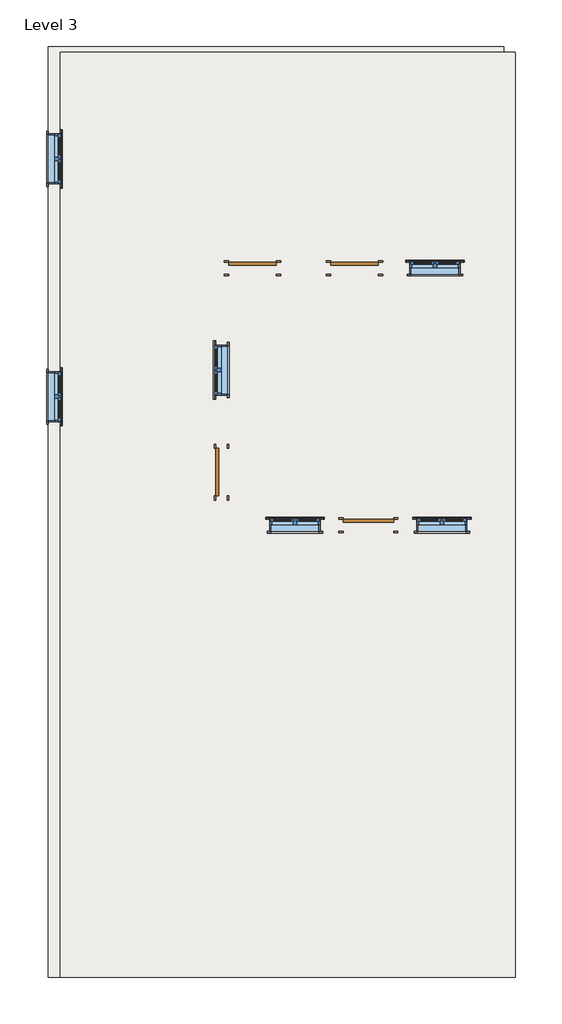
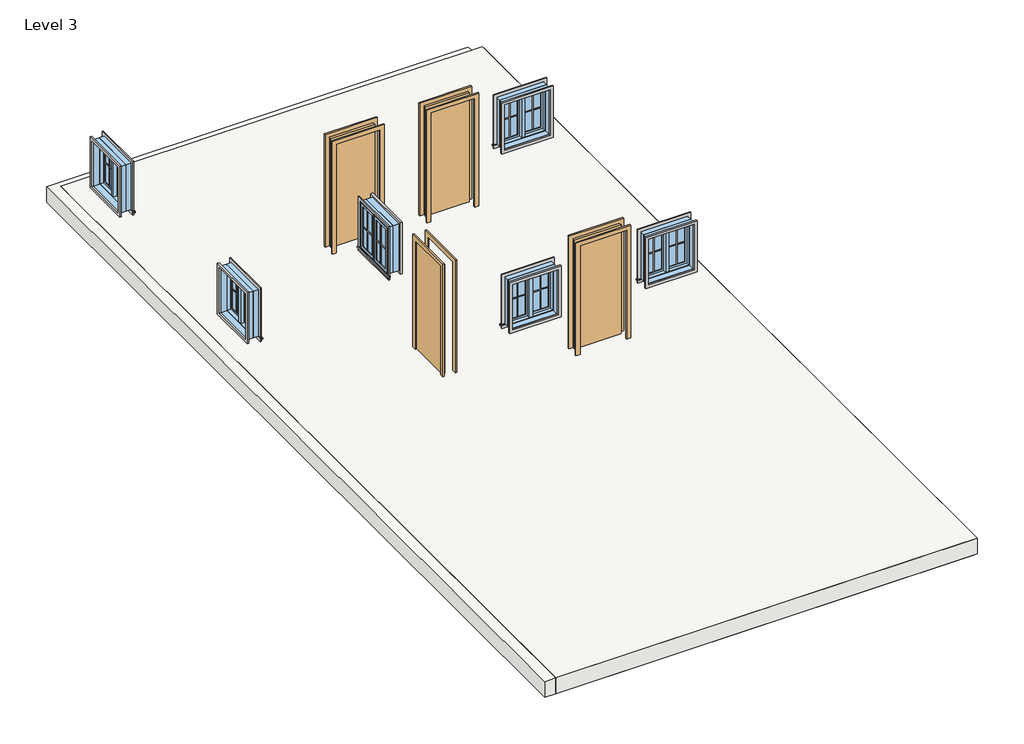
# One storey: 24 proxies, 6 windows, 4 doors, 4 slabs.
"""IFC4 building model written with IfcOpenShell, lengths in millimetres."""

from ifc_helpers import new_model, si_unit, frame, origin, place, context, project, spatial, polyline, outline, extrude, faceted_brep, transform, mapped, element, save
from components import muntin_pattern_2x2_muntin_pattern_2x2_b3fe6957, muntin_pattern_2x2_muntin_pattern_2x2_3e0ecaf2, trim_window_exterior_flat_with_sill_41619996, trim_window_interior_flat_picture_frame_51c85655, door_64d5ae29, door_f75d31f8, window_c29befe5

model = new_model("IFC4")

# Units and contexts
model_context = context("Model", 3, world=origin())
ifc_project = project(units=[si_unit("LENGTHUNIT", "METRE", prefix="MILLI")], contexts=[model_context])

# Site, building, storey
site = spatial("IfcSite", under=ifc_project)
building = spatial("IfcBuilding", under=site)
storey = spatial("IfcBuildingStorey", under=building, Name="Level 3", Elevation=12801.6)

# Proxies
placement = place(None, origin())
muntin_pattern_2x2_muntin_pattern_2x2_shape = muntin_pattern_2x2_muntin_pattern_2x2_b3fe6957(model_context)
element("IfcBuildingElementProxy", 1, Name="Muntin Pattern_2x2 : Muntin Pattern_2x2", ObjectType="Muntin Pattern_2x2 : Muntin Pattern_2x2", at=placement, inside=storey, context=model_context, shape_type="MappedRepresentation", body=[
    mapped(muntin_pattern_2x2_muntin_pattern_2x2_shape, transform((-15829.9638186, 14328.8576951, 13785.85), x_axis=(0.0, -1.0, 0.0), y_axis=(1.0, 0.0, 0.0), z_axis=(0.0, 0.0, 1.0))),
])
element("IfcBuildingElementProxy", 2, Name="Muntin Pattern_2x2 : Muntin Pattern_2x2", ObjectType="Muntin Pattern_2x2 : Muntin Pattern_2x2", at=placement, inside=storey, context=model_context, shape_type="MappedRepresentation", body=[
    mapped(muntin_pattern_2x2_muntin_pattern_2x2_shape, transform((-15829.9638186, 10239.4576951, 13785.85), x_axis=(0.0, -1.0, 0.0), y_axis=(1.0, 0.0, 0.0), z_axis=(0.0, 0.0, 1.0))),
])
element("IfcBuildingElementProxy", 3, Name="Muntin Pattern_2x2 : Muntin Pattern_2x2", ObjectType="Muntin Pattern_2x2 : Muntin Pattern_2x2", at=placement, inside=storey, context=model_context, shape_type="MappedRepresentation", body=[
    mapped(muntin_pattern_2x2_muntin_pattern_2x2_shape, transform((-9593.6723431, 12327.0201951, 13785.85), x_axis=(1.0, 0.0, 0.0), y_axis=(0.0, 1.0, 0.0), z_axis=(0.0, 0.0, 1.0))),
])
element("IfcBuildingElementProxy", 4, Name="Muntin Pattern_2x2 : Muntin Pattern_2x2", ObjectType="Muntin Pattern_2x2 : Muntin Pattern_2x2", at=placement, inside=storey, context=model_context, shape_type="MappedRepresentation", body=[
    mapped(muntin_pattern_2x2_muntin_pattern_2x2_shape, transform((-9474.1118308, 7907.4201951, 13785.85), x_axis=(1.0, 0.0, 0.0), y_axis=(0.0, 1.0, 0.0), z_axis=(0.0, 0.0, 1.0))),
])
element("IfcBuildingElementProxy", 5, Name="Muntin Pattern_2x2 : Muntin Pattern_2x2", ObjectType="Muntin Pattern_2x2 : Muntin Pattern_2x2", at=placement, inside=storey, context=model_context, shape_type="MappedRepresentation", body=[
    mapped(muntin_pattern_2x2_muntin_pattern_2x2_shape, transform((-11999.2328553, 7907.4201951, 13785.85), x_axis=(1.0, 0.0, 0.0), y_axis=(0.0, 1.0, 0.0), z_axis=(0.0, 0.0, 1.0))),
])
element("IfcBuildingElementProxy", 6, Name="Muntin Pattern_2x2 : Muntin Pattern_2x2", ObjectType="Muntin Pattern_2x2 : Muntin Pattern_2x2", at=placement, inside=storey, context=model_context, shape_type="MappedRepresentation", body=[
    mapped(muntin_pattern_2x2_muntin_pattern_2x2_shape, transform((-13139.5558676, 10268.0326951, 13785.85), x_axis=(0.0, 1.0, 0.0), y_axis=(-1.0, 0.0, 0.0), z_axis=(0.0, 0.0, 1.0))),
])
muntin_pattern_2x2_muntin_pattern_2x2_2_shape = muntin_pattern_2x2_muntin_pattern_2x2_3e0ecaf2(model_context)
element("IfcBuildingElementProxy", 7, Name="Muntin Pattern_2x2 : Muntin Pattern_2x2", ObjectType="Muntin Pattern_2x2 : Muntin Pattern_2x2", at=placement, inside=storey, context=model_context, shape_type="MappedRepresentation", body=[
    mapped(muntin_pattern_2x2_muntin_pattern_2x2_2_shape, transform((-15829.9638186, 13900.2326951, 13785.85), x_axis=(0.0, 1.0, 0.0), y_axis=(-1.0, 0.0, 0.0), z_axis=(0.0, 0.0, 1.0))),
])
element("IfcBuildingElementProxy", 8, Name="Muntin Pattern_2x2 : Muntin Pattern_2x2", ObjectType="Muntin Pattern_2x2 : Muntin Pattern_2x2", at=placement, inside=storey, context=model_context, shape_type="MappedRepresentation", body=[
    mapped(muntin_pattern_2x2_muntin_pattern_2x2_2_shape, transform((-15829.9638186, 9810.8326951, 13785.85), x_axis=(0.0, 1.0, 0.0), y_axis=(-1.0, 0.0, 0.0), z_axis=(0.0, 0.0, 1.0))),
])
element("IfcBuildingElementProxy", 9, Name="Muntin Pattern_2x2 : Muntin Pattern_2x2", ObjectType="Muntin Pattern_2x2 : Muntin Pattern_2x2", at=placement, inside=storey, context=model_context, shape_type="MappedRepresentation", body=[
    mapped(muntin_pattern_2x2_muntin_pattern_2x2_2_shape, transform((-9165.0473431, 12327.0201951, 13785.85), x_axis=(-1.0, 0.0, 0.0), y_axis=(0.0, -1.0, 0.0), z_axis=(0.0, 0.0, 1.0))),
])
element("IfcBuildingElementProxy", 10, Name="Muntin Pattern_2x2 : Muntin Pattern_2x2", ObjectType="Muntin Pattern_2x2 : Muntin Pattern_2x2", at=placement, inside=storey, context=model_context, shape_type="MappedRepresentation", body=[
    mapped(muntin_pattern_2x2_muntin_pattern_2x2_2_shape, transform((-9045.4868308, 7907.4201951, 13785.85), x_axis=(-1.0, 0.0, 0.0), y_axis=(0.0, -1.0, 0.0), z_axis=(0.0, 0.0, 1.0))),
])
element("IfcBuildingElementProxy", 11, Name="Muntin Pattern_2x2 : Muntin Pattern_2x2", ObjectType="Muntin Pattern_2x2 : Muntin Pattern_2x2", at=placement, inside=storey, context=model_context, shape_type="MappedRepresentation", body=[
    mapped(muntin_pattern_2x2_muntin_pattern_2x2_2_shape, transform((-11570.6078553, 7907.4201951, 13785.85), x_axis=(-1.0, 0.0, 0.0), y_axis=(0.0, -1.0, 0.0), z_axis=(0.0, 0.0, 1.0))),
])
element("IfcBuildingElementProxy", 12, Name="Muntin Pattern_2x2 : Muntin Pattern_2x2", ObjectType="Muntin Pattern_2x2 : Muntin Pattern_2x2", at=placement, inside=storey, context=model_context, shape_type="MappedRepresentation", body=[
    mapped(muntin_pattern_2x2_muntin_pattern_2x2_2_shape, transform((-13139.5558676, 10696.6576951, 13785.85), x_axis=(0.0, -1.0, 0.0), y_axis=(1.0, 0.0, 0.0), z_axis=(0.0, 0.0, 1.0))),
])
trim_window_exterior_flat_with_sill_shape = trim_window_exterior_flat_with_sill_41619996(model_context)
element("IfcBuildingElementProxy", 13, Name="Trim-Window-Exterior-Flat : with Sill", ObjectType="Trim-Window-Exterior-Flat : with Sill", at=placement, inside=storey, context=model_context, shape_type="MappedRepresentation", body=[
    mapped(trim_window_exterior_flat_with_sill_shape, transform((-15820.4388186, 14114.5451951, 14630.4), x_axis=(0.0, 1.0, 0.0), y_axis=(0.0, 0.0, 1.0), z_axis=(1.0, 0.0, 0.0))),
])
element("IfcBuildingElementProxy", 14, Name="Trim-Window-Exterior-Flat : with Sill", ObjectType="Trim-Window-Exterior-Flat : with Sill", at=placement, inside=storey, context=model_context, shape_type="MappedRepresentation", body=[
    mapped(trim_window_exterior_flat_with_sill_shape, transform((-15820.4388186, 10025.1451951, 14630.4), x_axis=(0.0, 1.0, 0.0), y_axis=(0.0, 0.0, 1.0), z_axis=(1.0, 0.0, 0.0))),
])
element("IfcBuildingElementProxy", 15, Name="Trim-Window-Exterior-Flat : with Sill", ObjectType="Trim-Window-Exterior-Flat : with Sill", at=placement, inside=storey, context=model_context, shape_type="MappedRepresentation", body=[
    mapped(trim_window_exterior_flat_with_sill_shape, transform((-9379.3598431, 12336.5451951, 14630.4), x_axis=(-1.0, 0.0, 0.0), y_axis=(0.0, 0.0, 1.0), z_axis=(0.0, 1.0, 0.0))),
])
element("IfcBuildingElementProxy", 16, Name="Trim-Window-Exterior-Flat : with Sill", ObjectType="Trim-Window-Exterior-Flat : with Sill", at=placement, inside=storey, context=model_context, shape_type="MappedRepresentation", body=[
    mapped(trim_window_exterior_flat_with_sill_shape, transform((-9259.7993308, 7916.9451951, 14630.4), x_axis=(-1.0, 0.0, 0.0), y_axis=(0.0, 0.0, 1.0), z_axis=(0.0, 1.0, 0.0))),
])
element("IfcBuildingElementProxy", 17, Name="Trim-Window-Exterior-Flat : with Sill", ObjectType="Trim-Window-Exterior-Flat : with Sill", at=placement, inside=storey, context=model_context, shape_type="MappedRepresentation", body=[
    mapped(trim_window_exterior_flat_with_sill_shape, transform((-11784.9203553, 7916.9451951, 14630.4), x_axis=(-1.0, 0.0, 0.0), y_axis=(0.0, 0.0, 1.0), z_axis=(0.0, 1.0, 0.0))),
])
element("IfcBuildingElementProxy", 18, Name="Trim-Window-Exterior-Flat : with Sill", ObjectType="Trim-Window-Exterior-Flat : with Sill", at=placement, inside=storey, context=model_context, shape_type="MappedRepresentation", body=[
    mapped(trim_window_exterior_flat_with_sill_shape, transform((-13149.0808676, 10482.3451951, 14630.4), x_axis=(0.0, -1.0, 0.0), y_axis=(0.0, 0.0, 1.0), z_axis=(-1.0, 0.0, 0.0))),
])
trim_window_interior_flat_picture_frame_shape = trim_window_interior_flat_picture_frame_51c85655(model_context)
element("IfcBuildingElementProxy", 19, Name="Trim-Window-Interior-Flat : Picture Frame", ObjectType="Trim-Window-Interior-Flat : Picture Frame", at=placement, inside=storey, context=model_context, shape_type="MappedRepresentation", body=[
    mapped(trim_window_interior_flat_picture_frame_shape, transform((-16023.6388186, 14114.5451951, 14630.4), x_axis=(0.0, -1.0, 0.0), y_axis=(0.0, 0.0, 1.0), z_axis=(-1.0, 0.0, 0.0))),
])
element("IfcBuildingElementProxy", 20, Name="Trim-Window-Interior-Flat : Picture Frame", ObjectType="Trim-Window-Interior-Flat : Picture Frame", at=placement, inside=storey, context=model_context, shape_type="MappedRepresentation", body=[
    mapped(trim_window_interior_flat_picture_frame_shape, transform((-16023.6388186, 10025.1451951, 14630.4), x_axis=(0.0, -1.0, 0.0), y_axis=(0.0, 0.0, 1.0), z_axis=(-1.0, 0.0, 0.0))),
])
element("IfcBuildingElementProxy", 21, Name="Trim-Window-Interior-Flat : Picture Frame", ObjectType="Trim-Window-Interior-Flat : Picture Frame", at=placement, inside=storey, context=model_context, shape_type="MappedRepresentation", body=[
    mapped(trim_window_interior_flat_picture_frame_shape, transform((-9379.3598431, 12133.3451951, 14630.4), x_axis=(1.0, 0.0, 0.0), y_axis=(0.0, 0.0, 1.0), z_axis=(0.0, -1.0, 0.0))),
])
element("IfcBuildingElementProxy", 22, Name="Trim-Window-Interior-Flat : Picture Frame", ObjectType="Trim-Window-Interior-Flat : Picture Frame", at=placement, inside=storey, context=model_context, shape_type="MappedRepresentation", body=[
    mapped(trim_window_interior_flat_picture_frame_shape, transform((-9259.7993308, 7713.7451951, 14630.4), x_axis=(1.0, 0.0, 0.0), y_axis=(0.0, 0.0, 1.0), z_axis=(0.0, -1.0, 0.0))),
])
element("IfcBuildingElementProxy", 23, Name="Trim-Window-Interior-Flat : Picture Frame", ObjectType="Trim-Window-Interior-Flat : Picture Frame", at=placement, inside=storey, context=model_context, shape_type="MappedRepresentation", body=[
    mapped(trim_window_interior_flat_picture_frame_shape, transform((-11784.9203553, 7713.7451951, 14630.4), x_axis=(1.0, 0.0, 0.0), y_axis=(0.0, 0.0, 1.0), z_axis=(0.0, -1.0, 0.0))),
])
element("IfcBuildingElementProxy", 24, Name="Trim-Window-Interior-Flat : Picture Frame", ObjectType="Trim-Window-Interior-Flat : Picture Frame", at=placement, inside=storey, context=model_context, shape_type="MappedRepresentation", body=[
    mapped(trim_window_interior_flat_picture_frame_shape, transform((-12945.8808676, 10482.3451951, 14630.4), x_axis=(0.0, 1.0, 0.0), y_axis=(0.0, 0.0, 1.0), z_axis=(1.0, 0.0, 0.0))),
])

# Doors
door_shape = door_64d5ae29(model_context)
element("IfcDoor", 25, ObjectType="Single-Flush : 32\" x 84\"", at=placement, inside=storey, context=model_context, shape_type="MappedRepresentation", body=[
    mapped(door_shape, transform((-12514.0808676, 12234.9451951, 12801.6), x_axis=(1.0, 0.0, 0.0), y_axis=(0.0, 1.0, 0.0), z_axis=(0.0, 0.0, 1.0))),
])
element("IfcDoor", 26, ObjectType="Single-Flush : 32\" x 84\"", at=placement, inside=storey, context=model_context, shape_type="MappedRepresentation", body=[
    mapped(door_shape, transform((-10761.4808676, 12234.9451951, 12801.6), x_axis=(1.0, 0.0, 0.0), y_axis=(0.0, 1.0, 0.0), z_axis=(0.0, 0.0, 1.0))),
])
element("IfcDoor", 27, ObjectType="Single-Flush : 32\" x 84\"", at=placement, inside=storey, context=model_context, shape_type="MappedRepresentation", body=[
    mapped(door_shape, transform((-13047.4808676, 8729.7451951, 12801.6), x_axis=(0.0, 1.0, 0.0), y_axis=(-1.0, 0.0, 0.0), z_axis=(0.0, 0.0, 1.0))),
])
door_2_shape = door_f75d31f8(model_context)
element("IfcDoor", 28, ObjectType="Single-Flush : 34\" x 84\"", at=placement, inside=storey, context=model_context, shape_type="MappedRepresentation", body=[
    mapped(door_2_shape, transform((-10522.3598431, 7815.3451951, 12801.6), x_axis=(1.0, 0.0, 0.0), y_axis=(0.0, 1.0, 0.0), z_axis=(0.0, 0.0, 1.0))),
])

# Slabs
element("IfcSlab", 29, ObjectType="Generic - 12\"", at=placement, inside=storey, context=model_context, shape_type="SweptSolid", body=[
    extrude(outline(polyline([(-7997.2388186, 15943.3451951), (-7997.2388186, 42.9451951), (-15820.4388186, 42.9451951), (-15820.4388186, 15943.3451951), (-7997.2388186, 15943.3451951)])), frame((0.0, 0.0, 12496.8), z_axis=(0.0, 0.0, 1.0), x_axis=(1.0, 0.0, 0.0)), (0.0, 0.0, 1.0), 304.8),
])
element("IfcSlab", 30, ObjectType="Generic - 12\"", at=placement, inside=storey, context=model_context, shape_type="Brep", body=[
    faceted_brep([(-7997.2388186, 15943.3451951, 12496.8), (-7997.2388186, 15892.5451951, 12496.8), (-7997.2388186, 42.9451951, 12496.8), (-8098.8388186, 42.9451951, 12496.8), (-15820.4388186, 42.9451951, 12496.8), (-15820.4388186, 15943.3451951, 12496.8), (-8200.4388186, 15943.3451951, 12496.8), (-8191.7229165, 15943.3451951, 12496.8), (-7997.2388186, 15943.3451951, 12801.6), (-8191.7229165, 15943.3451951, 12801.6), (-8200.4388186, 15943.3451951, 12801.6), (-15820.4388186, 15943.3451951, 12801.6), (-15820.4388186, 42.9451951, 12801.6), (-8098.8388186, 42.9451951, 12801.6), (-7997.2388186, 42.9451951, 12801.6), (-7997.2388186, 15892.5451951, 12801.6)], [[[0, 1, 2, 3, 4, 5, 6, 7]], [[8, 9, 10, 11, 12, 13, 14, 15]], [[2, 1, 0, 8, 15, 14]], [[4, 3, 2, 14, 13, 12]], [[5, 4, 12, 11]], [[0, 7, 6, 5, 11, 10, 9, 8]]]),
])
element("IfcSlab", 31, ObjectType="Generic - 12\"", at=placement, inside=storey, context=model_context, shape_type="Brep", body=[
    faceted_brep([(-7997.2388186, 15943.3451951, 12496.8), (-7997.2388186, 15892.5451951, 12496.8), (-7997.2388186, 42.9451951, 12496.8), (-8098.8388186, 42.9451951, 12496.8), (-15820.4388186, 42.9451951, 12496.8), (-15820.4388186, 15943.3451951, 12496.8), (-8200.4388186, 15943.3451951, 12496.8), (-8191.7229165, 15943.3451951, 12496.8), (-7997.2388186, 15943.3451951, 12801.6), (-8191.7229165, 15943.3451951, 12801.6), (-8200.4388186, 15943.3451951, 12801.6), (-15820.4388186, 15943.3451951, 12801.6), (-15820.4388186, 42.9451951, 12801.6), (-8098.8388186, 42.9451951, 12801.6), (-7997.2388186, 42.9451951, 12801.6), (-7997.2388186, 15892.5451951, 12801.6)], [[[0, 1, 2, 3, 4, 5, 6, 7]], [[8, 9, 10, 11, 12, 13, 14, 15]], [[2, 1, 0, 8, 15, 14]], [[4, 3, 2, 14, 13, 12]], [[5, 4, 12, 11]], [[0, 7, 6, 5, 11, 10, 9, 8]]]),
])
element("IfcSlab", 32, ObjectType="Generic - 12\"", at=placement, inside=storey, context=model_context, shape_type="Brep", body=[
    faceted_brep([(-8200.4388186, 16044.9451951, 12496.8), (-8200.4388186, 15952.0610972, 12496.8), (-8200.4388186, 15943.3451951, 12496.8), (-8200.4388186, 42.9451951, 12496.8), (-15820.4388186, 42.9451951, 12496.8), (-16023.6388186, 42.9451951, 12496.8), (-16023.6388186, 15892.5451951, 12496.8), (-16023.6388186, 16044.9451951, 12496.8), (-8293.3229165, 16044.9451951, 12496.8), (-8200.4388186, 16044.9451951, 12801.6), (-8293.3229165, 16044.9451951, 12801.6), (-16023.6388186, 16044.9451951, 12801.6), (-16023.6388186, 15892.5451951, 12801.6), (-16023.6388186, 42.9451951, 12801.6), (-15820.4388186, 42.9451951, 12801.6), (-8200.4388186, 42.9451951, 12801.6), (-8200.4388186, 15943.3451951, 12801.6), (-8200.4388186, 15952.0610972, 12801.6)], [[[0, 1, 2, 3, 4, 5, 6, 7, 8]], [[9, 10, 11, 12, 13, 14, 15, 16, 17]], [[3, 2, 1, 0, 9, 17, 16, 15]], [[5, 4, 3, 15, 14, 13]], [[7, 6, 5, 13, 12, 11]], [[0, 8, 7, 11, 10, 9]]]),
])

# Windows
window_shape = window_c29befe5(model_context)
element("IfcWindow", 33, ObjectType="Window-Casement-Double : 34\" x 36\"", at=placement, inside=storey, context=model_context, shape_type="MappedRepresentation", body=[
    mapped(window_shape, transform((-15922.0388186, 14114.5451951, 12801.6), x_axis=(0.0, -1.0, 0.0), y_axis=(1.0, 0.0, 0.0), z_axis=(0.0, 0.0, 1.0))),
])
element("IfcWindow", 34, ObjectType="Window-Casement-Double : 34\" x 36\"", at=placement, inside=storey, context=model_context, shape_type="MappedRepresentation", body=[
    mapped(window_shape, transform((-15922.0388186, 10025.1451951, 12801.6), x_axis=(0.0, -1.0, 0.0), y_axis=(1.0, 0.0, 0.0), z_axis=(0.0, 0.0, 1.0))),
])
element("IfcWindow", 35, ObjectType="Window-Casement-Double : 34\" x 36\"", at=placement, inside=storey, context=model_context, shape_type="MappedRepresentation", body=[
    mapped(window_shape, transform((-9379.3598431, 12234.9451951, 12801.6), x_axis=(1.0, 0.0, 0.0), y_axis=(0.0, 1.0, 0.0), z_axis=(0.0, 0.0, 1.0))),
])
element("IfcWindow", 36, ObjectType="Window-Casement-Double : 34\" x 36\"", at=placement, inside=storey, context=model_context, shape_type="MappedRepresentation", body=[
    mapped(window_shape, transform((-9259.7993308, 7815.3451951, 12801.6), x_axis=(1.0, 0.0, 0.0), y_axis=(0.0, 1.0, 0.0), z_axis=(0.0, 0.0, 1.0))),
])
element("IfcWindow", 37, ObjectType="Window-Casement-Double : 34\" x 36\"", at=placement, inside=storey, context=model_context, shape_type="MappedRepresentation", body=[
    mapped(window_shape, transform((-11784.9203553, 7815.3451951, 12801.6), x_axis=(1.0, 0.0, 0.0), y_axis=(0.0, 1.0, 0.0), z_axis=(0.0, 0.0, 1.0))),
])
element("IfcWindow", 38, ObjectType="Window-Casement-Double : 34\" x 36\"", at=placement, inside=storey, context=model_context, shape_type="MappedRepresentation", body=[
    mapped(window_shape, transform((-13047.4808676, 10482.3451951, 12801.6), x_axis=(0.0, 1.0, 0.0), y_axis=(-1.0, 0.0, 0.0), z_axis=(0.0, 0.0, 1.0))),
])

save(model, "model.ifc")

# Revit data of these elements
# Type "Muntin Pattern_2x2 : Muntin Pattern_2x2"
#   Width [instance default] = 4' - 0"
#   Thickness = 0' - 0 1/2"
#   Height [instance default] = 4' - 0"
#   Distance = 0' - 0 3/4"
#   Interior Material [instance default] = none
#   Exterior Material [instance default] = none
#   Default Elevation = 0
# Type "Trim-Window-Exterior-Flat : with Sill"
#   Trim Width = 0' - 2 1/4"
#   Trim Thickness_Picture Frame = 0' - 1 1/4"
#   Trim Thickness_with Sill = 0' - 0 3/4"
#   Sill Thickness = 0' - 1 1/4"
#   Opening Width [instance default] = 2' - 0"
#   Opening Height [instance default] = 3' - 0"
#   Default Elevation = 4' - 0"
#   Sill = yes
#   Picture Frame = no
#   Trim Material [instance default] = none
# Type "Trim-Window-Interior-Flat : Picture Frame"
#   Trim Thickness_Picture Frame = 0' - 1 1/4"
#   Trim Width = 0' - 2 1/4"
#   Trim Thickness_with Sill = 0' - 0 3/4"
#   Sill Thickness = 0' - 1 1/4"
#   Opening Width [instance default] = 2' - 0"
#   Opening Height [instance default] = 3' - 0"
#   Default Elevation = 4' - 0"
#   Sill = no
#   Picture Frame = yes
#   Trim Material [instance default] = none
# Type "Single-Flush : 32\" x 84\""
#   Type Mark = "3"
#   Construction Type Id = "MDOOR"
#   Assembly Code = "C1020"
#   Analytic Construction = "Metal"
#   Thickness = 0' - 2"
#   Heat Transfer Coefficient (U) = 0.651978 BTU/(h·ft²·°F)
#   Height = 7' - 0"
#   Trim Projection Ext = 0' - 1"
#   Trim Projection Int = 0' - 1"
#   Trim Width = 0' - 3"
#   Width = 2' - 8"
#   Define Thermal Properties by = 1
#   Define Thermal Properties by = 1
#   Door Material = Door - Panel
#   Frame Material = Door - Frame
#   Visual Light Transmittance = 0
#   Solar Heat Gain Coefficient = 0
#   Function = (empty or 0)
#   Wall Closure = (empty or 0)
# Type "Single-Flush : 34\" x 84\""
#   Type Mark = "2"
#   Construction Type Id = "MDOOR"
#   Assembly Code = "C1020"
#   Analytic Construction = "Metal"
#   Thickness = 0' - 2"
#   Heat Transfer Coefficient (U) = 0.651978 BTU/(h·ft²·°F)
#   Height = 7' - 0"
#   Trim Projection Ext = 0' - 1"
#   Trim Projection Int = 0' - 1"
#   Trim Width = 0' - 3"
#   Width = 2' - 10"
#   Define Thermal Properties by = 1
#   Define Thermal Properties by = 1
#   Door Material = Door - Panel
#   Frame Material = Door - Frame
#   Visual Light Transmittance = 0
#   Solar Heat Gain Coefficient = 0
#   Function = (empty or 0)
#   Wall Closure = (empty or 0)
# Type "Generic - 12\""
#   Assembly Code = "B1010"
#   Function = 0
#   Layers, outside or top first: 1' - 0" no material (function 1)
# Type "Window-Casement-Double : 34\" x 36\""
#   Type Mark = "14"
#   Fire Rating = "0.5h"
#   Assembly Code = "B2020100"
#   Analytic Construction = "Double glazing - domestic"
#   Frame Extension [instance default] = 0' - 0 1/4"
#   Window Inset [instance default] = 0' - 0"
#   Wall Thickness [instance default] = 0' - 6"
#   Interior Wall Closure [instance default] = 0' - 2 1/4"
#   Half Width = 1' - 5"
#   Visual Light Transmittance = 0.81
#   Thermal Resistance (R) = 1.8146 (h·ft²·°F)/BTU
#   Solar Heat Gain Coefficient = 0.76
#   Rough Width = 2' - 10 1/2"
#   Rough Height = 3' - 0 1/2"
#   Height = 3' - 0"
#   Heat Transfer Coefficient (U) = 0.5511 BTU/(h·ft²·°F)
#   Exterior Wall Closure [instance default] = 0' - 1 1/4"
#   Extension Jamb [instance default] = 0' - 2 1/4"
#   Default Sill Height = 3' - 0"
#   Width = 2' - 10"
#   Define Thermal Properties by = 0
#   Muntin Visibility = yes
#   Interior Trim Visibility [instance default] = yes
#   Exterior Trim Visibility [instance default] = yes
#   Extension Jamb Visibility [instance default] = yes
#   Interior Trim Material = Wood - Stained
#   Muntin Pattern = Muntin Pattern_2x2 : Muntin Pattern_2x2
#   Interior Trim = Trim-Window-Interior-Flat : Picture Frame
#   Interior Frame Material = Wood - Stained
#   Glass Panel Material = Glass
#   Exterior Trim Material = Clad - White
#   Exterior Trim = Trim-Window-Exterior-Flat : with Sill
#   Exterior Frame Material = Clad - White
#   Wall Closure = (empty or 0)
# Elements 1, 2, 3, 4, 5, 6, 7, 8, 9, 10, 11, 12 (IfcBuildingElementProxy, "Muntin Pattern_2x2 : Muntin Pattern_2x2")
#   Width = 0' - 11 5/8"
#   Height = 2' - 6 1/2"
#   Interior Material = Wood - Stained
#   Exterior Material = Clad - White
#   Phase Created = New Construction
#   Materials on its faces: "Clad - White", "Wood - Stained"
# Elements 13, 14, 15, 16, 17, 18 (IfcBuildingElementProxy, "Trim-Window-Exterior-Flat : with Sill")
#   Opening Width = 2' - 10"
#   Opening Height = 3' - 0"
#   Trim Material = Clad - White
#   Phase Created = New Construction
#   Materials on its faces: "Clad - White"
# Elements 19, 20, 21, 22, 23, 24 (IfcBuildingElementProxy, "Trim-Window-Interior-Flat : Picture Frame")
#   Opening Width = 2' - 10"
#   Opening Height = 3' - 0"
#   Trim Material = Wood - Stained
#   Phase Created = New Construction
#   Materials on its faces: "Wood - Stained"
# Elements 25, 26, 27 (IfcDoor, "Single-Flush : 32\" x 84\"")
#   Phase Created = New Construction
#   Materials on its faces: "Door - Frame", "Door - Panel"
# Element 28 (IfcDoor, "Single-Flush : 34\" x 84\"")
#   Phase Created = New Construction
#   Materials on its faces: "Door - Frame", "Door - Panel"
# Elements 29, 30, 31, 32 (IfcSlab, "Generic - 12\"")
#   Height Offset From Level = 0' - 0"
#   Phase Created = New Construction
#   Materials on its faces: "Default Floor"
# Element 33 (IfcWindow, "Window-Casement-Double : 34\" x 36\"")
#   Mark = "10"
#   Window Inset = 0' - 0"
#   Interior Wall Closure = 0' - 2 1/4"
#   Frame Extension = 0' - 0 1/4"
#   Exterior Wall Closure = 0' - 1 1/4"
#   Interior Trim Visibility = yes
#   Exterior Trim Visibility = yes
#   Phase Created = New Construction
#   Materials on its faces: "Wood - Stained", "Glass", "Clad - White"
# Element 34 (IfcWindow, "Window-Casement-Double : 34\" x 36\"")
#   Mark = "11"
#   Window Inset = 0' - 0"
#   Interior Wall Closure = 0' - 2 1/4"
#   Frame Extension = 0' - 0 1/4"
#   Exterior Wall Closure = 0' - 1 1/4"
#   Interior Trim Visibility = yes
#   Exterior Trim Visibility = yes
#   Phase Created = New Construction
#   Materials on its faces: "Wood - Stained", "Glass", "Clad - White"
# Element 35 (IfcWindow, "Window-Casement-Double : 34\" x 36\"")
#   Mark = "12"
#   Window Inset = 0' - 0"
#   Interior Wall Closure = 0' - 2 1/4"
#   Frame Extension = 0' - 0 1/4"
#   Exterior Wall Closure = 0' - 1 1/4"
#   Interior Trim Visibility = yes
#   Exterior Trim Visibility = yes
#   Phase Created = New Construction
#   Materials on its faces: "Wood - Stained", "Glass", "Clad - White"
# Element 36 (IfcWindow, "Window-Casement-Double : 34\" x 36\"")
#   Mark = "13"
#   Window Inset = 0' - 0"
#   Interior Wall Closure = 0' - 2 1/4"
#   Frame Extension = 0' - 0 1/4"
#   Exterior Wall Closure = 0' - 1 1/4"
#   Interior Trim Visibility = yes
#   Exterior Trim Visibility = yes
#   Phase Created = New Construction
#   Materials on its faces: "Wood - Stained", "Glass", "Clad - White"
# Element 37 (IfcWindow, "Window-Casement-Double : 34\" x 36\"")
#   Mark = "14"
#   Window Inset = 0' - 0"
#   Interior Wall Closure = 0' - 2 1/4"
#   Frame Extension = 0' - 0 1/4"
#   Exterior Wall Closure = 0' - 1 1/4"
#   Interior Trim Visibility = yes
#   Exterior Trim Visibility = yes
#   Phase Created = New Construction
#   Materials on its faces: "Wood - Stained", "Glass", "Clad - White"
# Element 38 (IfcWindow, "Window-Casement-Double : 34\" x 36\"")
#   Mark = "15"
#   Window Inset = 0' - 0"
#   Interior Wall Closure = 0' - 2 1/4"
#   Frame Extension = 0' - 0 1/4"
#   Exterior Wall Closure = 0' - 1 1/4"
#   Interior Trim Visibility = yes
#   Exterior Trim Visibility = yes
#   Phase Created = New Construction
#   Materials on its faces: "Wood - Stained", "Glass", "Clad - White"
# Materials
#   "Door - Panel": class "Wood", colour RGB 210 159 95, transparency 0, Cost = 0
#   "Door - Frame": colour RGB 118 70 51, transparency 0, Cost = 0
#   "Wood - Stained": class "Wood", colour RGB 224 178 126, transparency 0, Cost = 0
#   "Glass": class "Glass", colour RGB 0 128 192, transparency 0.75, Description = "Soda Lime Glass", Cost = 0
#   "Clad - White": class "Wood", colour RGB 242 242 238, transparency 0, Cost = 0
#   "Default Floor": colour RGB 128 128 128, transparency 0, Cost = 0
